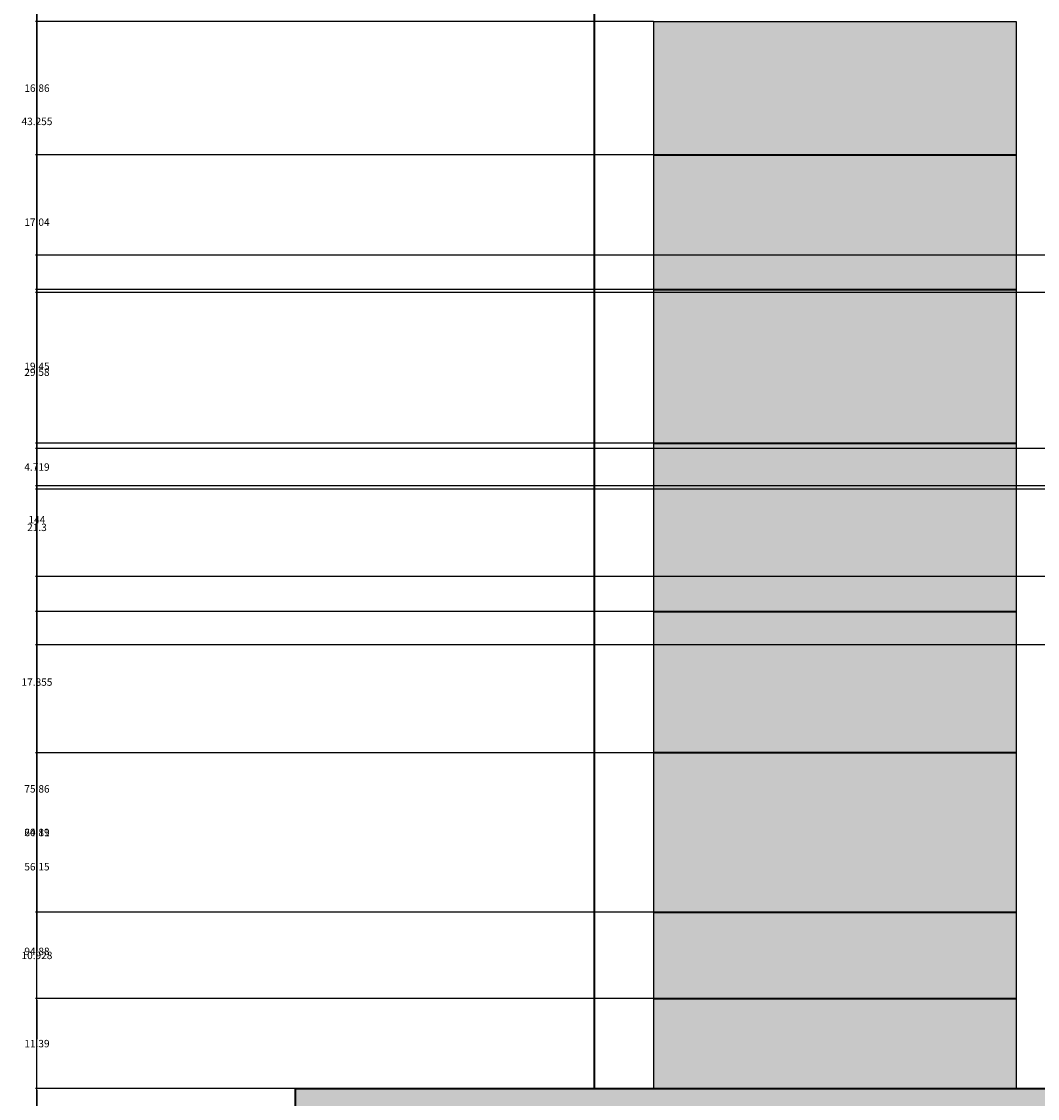
# Model space of a CAD drawing. Units: inches. Extents: x -5 to 714, y 84 to 644.
# Tile 2 of 20: x -5 to 124, y 200 to 336. Entities that reach past the tile are written whole.
import ezdxf

# ---------------------------------------------------------------- set-up
doc = ezdxf.new("R2010")
doc.units = ezdxf.units.IN
doc.header["$MEASUREMENT"] = 0
for name, color, linetype, lineweight in [('A-ANNO-DIMS', 2, 'Continuous', 18), ('A-ELEV', 7, 'Continuous', 35), ('A-ELEV-PATT', 8, 'Continuous', 13), ('A-GLAZ', 3, 'Continuous', 25)]:
    doc.layers.add(name, color=color, linetype=linetype, lineweight=lineweight)
doc.styles.get("Standard").update_dxf_attribs({"font": 'arial.ttf'})
doc.dimstyles.get("Standard").update_dxf_attribs({"dimtxt": 0.9375, "dimasz": 0.18, "dimexe": 0.18, "dimexo": 0.0625, "dimgap": 0.09, "dimtad": 0, "dimtih": 1, "dimtoh": 1, "dimdec": 4, "dimzin": 0, "dimdsep": 46, "dimlunit": 4, "dimtxsty": 'Standard', "dimcen": 0.09, "dimadec": 0, "dimazin": 0, "dimtfac": 1, "dimtdec": 4, "dimtofl": 0, "dimtmove": 0, "dimatfit": 3, "dimfxl": 1, "dimtolj": 1, "dimtzin": 0, "dimarcsym": 0})

# ---------------------------------------------------------------- blocks, each defined once
blk = doc.blocks.new('*D2')
at = {"layer": 'A-ANNO-DIMS', "color": 0, "lineweight": -2, "transparency": 16777216}
for p, q in [((67.93, 610.73), (-2.74, 610.73)), ((-2.56, 610.55), (-2.56, 364.53)), ((-2.56, 117.37), (-2.56, 363.39)), ((30.08, 117.19), (-2.74, 117.19))]:
    blk.add_line(p, q, dxfattribs=at)
at = {"layer": 'A-ANNO-DIMS', "color": 0, "transparency": 16777216}
for points in [[(-2.59, 610.55), (-2.53, 610.55), (-2.56, 610.73)], [(-2.59, 117.37), (-2.53, 117.37), (-2.56, 117.19)]]:
    blk.add_solid(points, dxfattribs=at)
at = {"layer": 'Defpoints', "color": 0, "transparency": 16777216}
for p in [(-2.56, 610.73), (67.99, 610.73), (30.14, 117.19)]:
    blk.add_point(p, dxfattribs=at)
at = {"layer": 'A-ANNO-DIMS', "color": 0, "transparency": 16777216, "insert": (-2.56, 363.96), "char_height": 0.938, "attachment_point": 5}
blk.add_mtext('\\A1;493.5', dxfattribs=at)
blk = doc.blocks.new('*D4')
at = {"layer": 'A-ANNO-DIMS', "color": 0, "lineweight": -2, "transparency": 16777216}
for p, q in [((30.08, 201.19), (-2.74, 201.19)), ((-2.56, 201.01), (-2.56, 171.76)), ((-2.56, 141.37), (-2.56, 170.62)), ((30.08, 141.19), (-2.74, 141.19))]:
    blk.add_line(p, q, dxfattribs=at)
at = {"layer": 'A-ANNO-DIMS', "color": 0, "transparency": 16777216}
for points in [[(-2.59, 201.01), (-2.53, 201.01), (-2.56, 201.19)], [(-2.59, 141.37), (-2.53, 141.37), (-2.56, 141.19)]]:
    blk.add_solid(points, dxfattribs=at)
at = {"layer": 'Defpoints', "color": 0, "transparency": 16777216}
for p in [(-2.56, 201.19), (30.14, 201.19), (30.14, 141.19)]:
    blk.add_point(p, dxfattribs=at)
at = {"layer": 'A-ANNO-DIMS', "color": 0, "transparency": 16777216, "insert": (-2.56, 171.19), "char_height": 0.938, "attachment_point": 5}
blk.add_mtext('\\A1;60', dxfattribs=at)
blk = doc.blocks.new('*D5')
at = {"layer": 'A-ANNO-DIMS', "color": 0, "lineweight": -2, "transparency": 16777216}
for p, q in [((67.93, 345.19), (-2.74, 345.19)), ((-2.56, 345.01), (-2.56, 273.75)), ((-2.56, 201.37), (-2.56, 272.63)), ((67.93, 201.19), (-2.74, 201.19))]:
    blk.add_line(p, q, dxfattribs=at)
at = {"layer": 'A-ANNO-DIMS', "color": 0, "transparency": 16777216}
for points in [[(-2.59, 345.01), (-2.53, 345.01), (-2.56, 345.19)], [(-2.59, 201.37), (-2.53, 201.37), (-2.56, 201.19)]]:
    blk.add_solid(points, dxfattribs=at)
at = {"layer": 'Defpoints', "color": 0, "transparency": 16777216}
for p in [(-2.56, 345.19), (67.99, 345.19), (67.99, 201.19)]:
    blk.add_point(p, dxfattribs=at)
at = {"layer": 'A-ANNO-DIMS', "color": 0, "transparency": 16777216, "insert": (-2.56, 273.19), "char_height": 0.938, "attachment_point": 5}
blk.add_mtext('\\A1;144', dxfattribs=at)
blk = doc.blocks.new('*D38')
at = {"layer": 'A-ANNO-DIMS', "color": 0, "lineweight": -2, "transparency": 16777216}
for p, q in [((75.44, 212.58), (-2.74, 212.58)), ((-2.56, 212.4), (-2.56, 207.46)), ((-2.56, 201.37), (-2.56, 206.32)), ((75.44, 201.19), (-2.74, 201.19))]:
    blk.add_line(p, q, dxfattribs=at)
at = {"layer": 'A-ANNO-DIMS', "color": 0, "transparency": 16777216}
for points in [[(-2.59, 212.4), (-2.53, 212.4), (-2.56, 212.58)], [(-2.59, 201.37), (-2.53, 201.37), (-2.56, 201.19)]]:
    blk.add_solid(points, dxfattribs=at)
at = {"layer": 'Defpoints', "color": 0, "transparency": 16777216}
for p in [(-2.56, 212.58), (75.5, 212.58), (75.5, 201.19)]:
    blk.add_point(p, dxfattribs=at)
at = {"layer": 'A-ANNO-DIMS', "color": 0, "transparency": 16777216, "insert": (-2.56, 206.89), "char_height": 0.938, "attachment_point": 5}
blk.add_mtext('\\A1;11.39', dxfattribs=at)
blk = doc.blocks.new('*D39')
at = {"layer": 'A-ANNO-DIMS', "color": 0, "lineweight": -2, "transparency": 16777216}
for p, q in [((75.44, 223.51), (-2.74, 223.51)), ((-2.56, 223.33), (-2.56, 218.62)), ((-2.56, 212.76), (-2.56, 217.48)), ((75.44, 212.58), (-2.74, 212.58))]:
    blk.add_line(p, q, dxfattribs=at)
at = {"layer": 'A-ANNO-DIMS', "color": 0, "transparency": 16777216}
for points in [[(-2.59, 223.33), (-2.53, 223.33), (-2.56, 223.51)], [(-2.59, 212.76), (-2.53, 212.76), (-2.56, 212.58)]]:
    blk.add_solid(points, dxfattribs=at)
at = {"layer": 'Defpoints', "color": 0, "transparency": 16777216}
for p in [(-2.56, 223.51), (75.5, 223.51), (75.5, 212.58)]:
    blk.add_point(p, dxfattribs=at)
at = {"layer": 'A-ANNO-DIMS', "color": 0, "transparency": 16777216, "insert": (-2.56, 218.05), "char_height": 0.938, "attachment_point": 5}
blk.add_mtext('\\A1;10.928', dxfattribs=at)
blk = doc.blocks.new('*D40')
at = {"layer": 'A-ANNO-DIMS', "color": 0, "lineweight": -2, "transparency": 16777216}
for p, q in [((75.44, 243.7), (-2.74, 243.7)), ((-2.56, 243.52), (-2.56, 234.17)), ((-2.56, 223.69), (-2.56, 233.04)), ((75.44, 223.51), (-2.74, 223.51))]:
    blk.add_line(p, q, dxfattribs=at)
at = {"layer": 'A-ANNO-DIMS', "color": 0, "transparency": 16777216}
for points in [[(-2.59, 243.52), (-2.53, 243.52), (-2.56, 243.7)], [(-2.59, 223.69), (-2.53, 223.69), (-2.56, 223.51)]]:
    blk.add_solid(points, dxfattribs=at)
at = {"layer": 'Defpoints', "color": 0, "transparency": 16777216}
for p in [(-2.56, 243.7), (75.5, 243.7), (75.5, 223.51)]:
    blk.add_point(p, dxfattribs=at)
at = {"layer": 'A-ANNO-DIMS', "color": 0, "transparency": 16777216, "insert": (-2.56, 233.61), "char_height": 0.938, "attachment_point": 5}
blk.add_mtext('\\A1;20.19', dxfattribs=at)
blk = doc.blocks.new('*D41')
at = {"layer": 'A-ANNO-DIMS', "color": 0, "lineweight": -2, "transparency": 16777216}
for p, q in [((75.44, 261.56), (-2.74, 261.56)), ((-2.56, 261.38), (-2.56, 253.2)), ((-2.56, 243.88), (-2.56, 252.06)), ((75.44, 243.7), (-2.74, 243.7))]:
    blk.add_line(p, q, dxfattribs=at)
at = {"layer": 'A-ANNO-DIMS', "color": 0, "transparency": 16777216}
for points in [[(-2.59, 261.38), (-2.53, 261.38), (-2.56, 261.56)], [(-2.59, 243.88), (-2.53, 243.88), (-2.56, 243.7)]]:
    blk.add_solid(points, dxfattribs=at)
at = {"layer": 'Defpoints', "color": 0, "transparency": 16777216}
for p in [(-2.56, 261.56), (75.5, 261.56), (75.5, 243.7)]:
    blk.add_point(p, dxfattribs=at)
at = {"layer": 'A-ANNO-DIMS', "color": 0, "transparency": 16777216, "insert": (-2.56, 252.63), "char_height": 0.938, "attachment_point": 5}
blk.add_mtext('\\A1;17.855', dxfattribs=at)
blk = doc.blocks.new('*D42')
at = {"layer": 'A-ANNO-DIMS', "color": 0, "lineweight": -2, "transparency": 16777216}
for p, q in [((75.44, 282.86), (-2.74, 282.86)), ((-2.56, 282.68), (-2.56, 272.77)), ((-2.56, 261.74), (-2.56, 271.64)), ((75.44, 261.56), (-2.74, 261.56))]:
    blk.add_line(p, q, dxfattribs=at)
at = {"layer": 'A-ANNO-DIMS', "color": 0, "transparency": 16777216}
for points in [[(-2.59, 282.68), (-2.53, 282.68), (-2.56, 282.86)], [(-2.59, 261.74), (-2.53, 261.74), (-2.56, 261.56)]]:
    blk.add_solid(points, dxfattribs=at)
at = {"layer": 'Defpoints', "color": 0, "transparency": 16777216}
for p in [(-2.56, 282.86), (75.5, 282.86), (75.5, 261.56)]:
    blk.add_point(p, dxfattribs=at)
at = {"layer": 'A-ANNO-DIMS', "color": 0, "transparency": 16777216, "insert": (-2.56, 272.21), "char_height": 0.938, "attachment_point": 5}
blk.add_mtext('\\A1;21.3', dxfattribs=at)
blk = doc.blocks.new('*D43')
at = {"layer": 'A-ANNO-DIMS', "color": 0, "lineweight": -2, "transparency": 16777216}
for p, q in [((75.44, 302.3), (-2.74, 302.3)), ((-2.56, 302.12), (-2.56, 293.15)), ((-2.56, 283.04), (-2.56, 292.01)), ((75.44, 282.86), (-2.74, 282.86))]:
    blk.add_line(p, q, dxfattribs=at)
at = {"layer": 'A-ANNO-DIMS', "color": 0, "transparency": 16777216}
for points in [[(-2.59, 302.12), (-2.53, 302.12), (-2.56, 302.3)], [(-2.59, 283.04), (-2.53, 283.04), (-2.56, 282.86)]]:
    blk.add_solid(points, dxfattribs=at)
at = {"layer": 'Defpoints', "color": 0, "transparency": 16777216}
for p in [(-2.56, 302.3), (75.5, 302.3), (75.5, 282.86)]:
    blk.add_point(p, dxfattribs=at)
at = {"layer": 'A-ANNO-DIMS', "color": 0, "transparency": 16777216, "insert": (-2.56, 292.58), "char_height": 0.938, "attachment_point": 5}
blk.add_mtext('\\A1;19.45', dxfattribs=at)
blk = doc.blocks.new('*D44')
at = {"layer": 'A-ANNO-DIMS', "color": 0, "lineweight": -2, "transparency": 16777216}
for p, q in [((75.44, 319.34), (-2.74, 319.34)), ((-2.56, 319.16), (-2.56, 311.39)), ((-2.56, 302.48), (-2.56, 310.26)), ((75.44, 302.3), (-2.74, 302.3))]:
    blk.add_line(p, q, dxfattribs=at)
at = {"layer": 'A-ANNO-DIMS', "color": 0, "transparency": 16777216}
for points in [[(-2.59, 319.16), (-2.53, 319.16), (-2.56, 319.34)], [(-2.59, 302.48), (-2.53, 302.48), (-2.56, 302.3)]]:
    blk.add_solid(points, dxfattribs=at)
at = {"layer": 'Defpoints', "color": 0, "transparency": 16777216}
for p in [(-2.56, 319.34), (75.5, 319.34), (75.5, 302.3)]:
    blk.add_point(p, dxfattribs=at)
at = {"layer": 'A-ANNO-DIMS', "color": 0, "transparency": 16777216, "insert": (-2.56, 310.82), "char_height": 0.938, "attachment_point": 5}
blk.add_mtext('\\A1;17.04', dxfattribs=at)
blk = doc.blocks.new('*D45')
at = {"layer": 'A-ANNO-DIMS', "color": 0, "lineweight": -2, "transparency": 16777216}
for p, q in [((75.44, 336.21), (-2.74, 336.21)), ((-2.56, 336.03), (-2.56, 328.34)), ((-2.56, 319.52), (-2.56, 327.21)), ((75.44, 319.34), (-2.74, 319.34))]:
    blk.add_line(p, q, dxfattribs=at)
at = {"layer": 'A-ANNO-DIMS', "color": 0, "transparency": 16777216}
for points in [[(-2.59, 336.03), (-2.53, 336.03), (-2.56, 336.21)], [(-2.59, 319.52), (-2.53, 319.52), (-2.56, 319.34)]]:
    blk.add_solid(points, dxfattribs=at)
at = {"layer": 'Defpoints', "color": 0, "transparency": 16777216}
for p in [(-2.56, 336.21), (75.5, 336.21), (75.5, 319.34)]:
    blk.add_point(p, dxfattribs=at)
at = {"layer": 'A-ANNO-DIMS', "color": 0, "transparency": 16777216, "insert": (-2.56, 327.78), "char_height": 0.938, "attachment_point": 5}
blk.add_mtext('\\A1;16.86', dxfattribs=at)
blk = doc.blocks.new('*D50')
at = {"layer": 'A-ANNO-DIMS', "color": 0, "lineweight": -2, "transparency": 16777216}
for p, q in [((200.67, 345.19), (-2.74, 345.19)), ((-2.56, 345.01), (-2.56, 324.13)), ((-2.56, 302.12), (-2.56, 323)), ((200.67, 301.94), (-2.74, 301.94))]:
    blk.add_line(p, q, dxfattribs=at)
at = {"layer": 'A-ANNO-DIMS', "color": 0, "transparency": 16777216}
for points in [[(-2.59, 345.01), (-2.53, 345.01), (-2.56, 345.19)], [(-2.59, 302.12), (-2.53, 302.12), (-2.56, 301.94)]]:
    blk.add_solid(points, dxfattribs=at)
at = {"layer": 'Defpoints', "color": 0, "transparency": 16777216}
for p in [(-2.56, 345.19), (200.74, 345.19), (200.74, 301.94)]:
    blk.add_point(p, dxfattribs=at)
at = {"layer": 'A-ANNO-DIMS', "color": 0, "transparency": 16777216, "insert": (-2.56, 323.57), "char_height": 0.938, "attachment_point": 5}
blk.add_mtext('\\A1;43.255', dxfattribs=at)
blk = doc.blocks.new('*D56')
at = {"layer": 'A-ANNO-DIMS', "color": 0, "lineweight": -2, "transparency": 16777216}
for p, q in [((578.03, 277.05), (-2.74, 277.05)), ((-2.56, 276.87), (-2.56, 239.69)), ((-2.56, 201.37), (-2.56, 238.55)), ((578.03, 201.19), (-2.74, 201.19))]:
    blk.add_line(p, q, dxfattribs=at)
at = {"layer": 'A-ANNO-DIMS', "color": 0, "transparency": 16777216}
for points in [[(-2.59, 276.87), (-2.53, 276.87), (-2.56, 277.05)], [(-2.59, 201.37), (-2.53, 201.37), (-2.56, 201.19)]]:
    blk.add_solid(points, dxfattribs=at)
at = {"layer": 'Defpoints', "color": 0, "transparency": 16777216}
for p in [(-2.56, 277.05), (578.09, 277.05), (578.09, 201.19)]:
    blk.add_point(p, dxfattribs=at)
at = {"layer": 'A-ANNO-DIMS', "color": 0, "transparency": 16777216, "insert": (-2.56, 239.12), "char_height": 0.938, "attachment_point": 5}
blk.add_mtext('\\A1;75.86', dxfattribs=at)
blk = doc.blocks.new('*D57')
at = {"layer": 'A-ANNO-DIMS', "color": 0, "lineweight": -2, "transparency": 16777216}
for p, q in [((578.03, 306.63), (-2.74, 306.63)), ((-2.56, 306.45), (-2.56, 292.41)), ((-2.56, 277.23), (-2.56, 291.27)), ((578.03, 277.05), (-2.74, 277.05))]:
    blk.add_line(p, q, dxfattribs=at)
at = {"layer": 'A-ANNO-DIMS', "color": 0, "transparency": 16777216}
for points in [[(-2.59, 306.45), (-2.53, 306.45), (-2.56, 306.63)], [(-2.59, 277.23), (-2.53, 277.23), (-2.56, 277.05)]]:
    blk.add_solid(points, dxfattribs=at)
at = {"layer": 'Defpoints', "color": 0, "transparency": 16777216}
for p in [(578.09, 306.63), (-2.56, 277.05), (578.09, 277.05)]:
    blk.add_point(p, dxfattribs=at)
at = {"layer": 'A-ANNO-DIMS', "color": 0, "transparency": 16777216, "insert": (-2.56, 291.84), "char_height": 0.938, "attachment_point": 5}
blk.add_mtext('\\A1;29.58', dxfattribs=at)
blk = doc.blocks.new('*D59')
at = {"layer": 'A-ANNO-DIMS', "color": 0, "lineweight": -2, "transparency": 16777216}
for p, q in [((593.37, 282.2), (-2.74, 282.2)), ((-2.56, 282.02), (-2.56, 280.41)), ((-2.56, 277.66), (-2.56, 279.27)), ((593.37, 277.48), (-2.74, 277.48))]:
    blk.add_line(p, q, dxfattribs=at)
at = {"layer": 'A-ANNO-DIMS', "color": 0, "transparency": 16777216}
for points in [[(-2.59, 282.02), (-2.53, 282.02), (-2.56, 282.2)], [(-2.59, 277.66), (-2.53, 277.66), (-2.56, 277.48)]]:
    blk.add_solid(points, dxfattribs=at)
at = {"layer": 'Defpoints', "color": 0, "transparency": 16777216}
for p in [(-2.56, 282.2), (593.43, 282.2), (593.43, 277.48)]:
    blk.add_point(p, dxfattribs=at)
at = {"layer": 'A-ANNO-DIMS', "color": 0, "transparency": 16777216, "insert": (-2.56, 279.84), "char_height": 0.938, "attachment_point": 5}
blk.add_mtext('\\A1;4.719', dxfattribs=at)
blk = doc.blocks.new('*D65')
at = {"layer": 'A-ANNO-DIMS', "color": 0, "lineweight": -2, "transparency": 16777216}
for p, q in [((325.77, 266), (-2.74, 266)), ((-2.56, 265.82), (-2.56, 219.13)), ((-2.56, 171.3), (-2.56, 217.99)), ((325.77, 171.12), (-2.74, 171.12))]:
    blk.add_line(p, q, dxfattribs=at)
at = {"layer": 'A-ANNO-DIMS', "color": 0, "transparency": 16777216}
for points in [[(-2.59, 265.82), (-2.53, 265.82), (-2.56, 266)], [(-2.59, 171.3), (-2.53, 171.3), (-2.56, 171.12)]]:
    blk.add_solid(points, dxfattribs=at)
at = {"layer": 'Defpoints', "color": 0, "transparency": 16777216}
for p in [(-2.56, 266), (325.83, 266), (325.83, 171.12)]:
    blk.add_point(p, dxfattribs=at)
at = {"layer": 'A-ANNO-DIMS', "color": 0, "transparency": 16777216, "insert": (-2.56, 218.56), "char_height": 0.938, "attachment_point": 5}
blk.add_mtext('\\A1;94.88', dxfattribs=at)
blk = doc.blocks.new('*D71')
at = {"layer": 'A-ANNO-DIMS', "color": 0, "lineweight": -2, "transparency": 16777216}
for p, q in [((537.12, 257.34), (-2.74, 257.34)), ((-2.56, 257.16), (-2.56, 229.83)), ((-2.56, 201.37), (-2.56, 228.7)), ((537.12, 201.19), (-2.74, 201.19))]:
    blk.add_line(p, q, dxfattribs=at)
at = {"layer": 'A-ANNO-DIMS', "color": 0, "transparency": 16777216}
for points in [[(-2.59, 257.16), (-2.53, 257.16), (-2.56, 257.34)], [(-2.59, 201.37), (-2.53, 201.37), (-2.56, 201.19)]]:
    blk.add_solid(points, dxfattribs=at)
at = {"layer": 'Defpoints', "color": 0, "transparency": 16777216}
for p in [(-2.56, 257.34), (537.18, 257.34), (537.18, 201.19)]:
    blk.add_point(p, dxfattribs=at)
at = {"layer": 'A-ANNO-DIMS', "color": 0, "transparency": 16777216, "insert": (-2.56, 229.27), "char_height": 0.938, "attachment_point": 5}
blk.add_mtext('\\A1;56.15', dxfattribs=at)
blk = doc.blocks.new('*D72')
at = {"layer": 'A-ANNO-DIMS', "color": 0, "lineweight": -2, "transparency": 16777216}
for p, q in [((493.71, 266), (-2.74, 266)), ((-2.56, 265.82), (-2.56, 234.17)), ((-2.56, 201.37), (-2.56, 233.03)), ((493.71, 201.19), (-2.74, 201.19))]:
    blk.add_line(p, q, dxfattribs=at)
at = {"layer": 'A-ANNO-DIMS', "color": 0, "transparency": 16777216}
for points in [[(-2.59, 265.82), (-2.53, 265.82), (-2.56, 266)], [(-2.59, 201.37), (-2.53, 201.37), (-2.56, 201.19)]]:
    blk.add_solid(points, dxfattribs=at)
at = {"layer": 'Defpoints', "color": 0, "transparency": 16777216}
for p in [(-2.56, 266), (493.78, 266), (493.78, 201.19)]:
    blk.add_point(p, dxfattribs=at)
at = {"layer": 'A-ANNO-DIMS', "color": 0, "transparency": 16777216, "insert": (-2.56, 233.6), "char_height": 0.938, "attachment_point": 5}
blk.add_mtext('\\A1;64.81', dxfattribs=at)
blk = doc.blocks.new('*D82')
at = {"layer": 'A-ANNO-DIMS', "color": 0, "lineweight": -2, "transparency": 16777216}
for p, q in [((263.37, 201.19), (-2.74, 201.19)), ((-2.56, 201.01), (-2.56, 177.22)), ((-2.56, 152.3), (-2.56, 176.09)), ((263.37, 152.12), (-2.74, 152.12))]:
    blk.add_line(p, q, dxfattribs=at)
at = {"layer": 'A-ANNO-DIMS', "color": 0, "transparency": 16777216}
for points in [[(-2.59, 201.01), (-2.53, 201.01), (-2.56, 201.19)], [(-2.59, 152.3), (-2.53, 152.3), (-2.56, 152.12)]]:
    blk.add_solid(points, dxfattribs=at)
at = {"layer": 'Defpoints', "color": 0, "transparency": 16777216}
for p in [(-2.56, 201.19), (263.43, 201.19), (263.43, 152.12)]:
    blk.add_point(p, dxfattribs=at)
at = {"layer": 'A-ANNO-DIMS', "color": 0, "transparency": 16777216, "insert": (-2.56, 176.66), "char_height": 0.938, "attachment_point": 5}
blk.add_mtext('\\A1;49.08', dxfattribs=at)

msp = doc.modelspace()

# ---------------------------------------------------------------- hatches: boundary and pattern name
at = {"layer": 'A-ELEV-PATT', "transparency": 33554687}
h = msp.add_hatch(color=256, dxfattribs=at)
h.dxf.hatch_style = 1
h.paths.add_polyline_path([(188.3677, 525.1928), (67.9893, 525.1928), (67.9893, 489.1928), (67.9893, 345.1928), (126.7303, 345.1928), (126.7303, 480.1709), (229.3575, 480.1709), (229.3575, 525.1928), (212.6043, 525.1928), (212.6043, 482.7164), (211.0019, 482.7164), (211.0019, 525.1928), (207.6919, 525.1928), (199.9852, 525.1928), (199.9852, 482.7164), (198.3828, 482.7164), (198.3828, 525.1928), (189.9701, 525.1928), (189.9701, 482.7164), (188.3677, 482.7164)])
h.paths.add_polyline_path([(121.3589, 336.2066), (75.5048, 336.2066), (75.5048, 319.345), (121.3589, 319.345)])
h.paths.add_polyline_path([(121.3589, 319.345), (75.5048, 319.345), (75.5048, 302.3045), (121.3589, 302.3045)])
h.paths.add_polyline_path([(121.3589, 302.3045), (75.5048, 302.3045), (75.5048, 282.8561), (121.3589, 282.8561)])
h.paths.add_polyline_path([(121.3589, 282.8561), (75.5048, 282.8561), (75.5048, 261.5556), (121.3589, 261.5556)])
h.paths.add_polyline_path([(121.3589, 261.5556), (75.5048, 261.5556), (75.5048, 243.7009), (121.3589, 243.7009)])
h.paths.add_polyline_path([(121.3589, 243.7009), (75.5048, 243.7009), (75.5048, 223.5117), (121.3589, 223.5117)])
h.paths.add_polyline_path([(121.3589, 223.5117), (75.5048, 223.5117), (75.5048, 212.5836), (121.3589, 212.5836)])
h.paths.add_polyline_path([(121.3589, 212.5836), (75.5048, 212.5836), (75.5048, 201.1928), (121.3589, 201.1928)])
h.paths.add_polyline_path([(179.9335, 201.1928), (30.1395, 201.1928), (30.1395, 198.7054), (179.9335, 198.7054)])
h.paths.add_polyline_path([(187.6349, 201.1928), (179.9335, 201.1928), (179.9335, 198.7054), (179.9335, 141.1928), (269.2446, 141.1928), (269.2446, 201.1928), (263.4349, 201.1928), (263.4349, 152.1176), (187.6349, 152.1176)])
h.paths.add_polyline_path([(269.2446, 277.0513), (269.2446, 287.501), (269.2446, 306.6286), (578.0915, 306.6286), (578.0915, 201.1928), (593.428, 201.1928), (593.428, 315.0968), (584.4202, 315.0968), (259.0665, 315.0968), (259.0665, 201.1928), (263.4349, 201.1928), (269.2446, 201.1928)])

# ---------------------------------------------------------------- linework, layer by layer
at = {"layer": 'A-ELEV'}
for p, q in [((67.9893, 201.1928), (67.9893, 345.1928)), ((75.5048, 319.345), (121.3589, 319.345)), ((75.5048, 302.3045), (121.3589, 302.3045)), ((75.5048, 282.8561), (121.3589, 282.8561)), ((75.5048, 261.5556), (121.3589, 261.5556)), ((75.5048, 243.7009), (121.3589, 243.7009)), ((75.5048, 223.5117), (121.3589, 223.5117)), ((75.5048, 212.5836), (121.3589, 212.5836)), ((30.1395, 141.1928), (30.1395, 201.1928)), ((30.1395, 201.1928), (545.1065, 201.1928))]:
    msp.add_line(p, q, dxfattribs=at)
at = {"layer": 'A-GLAZ'}
msp.add_lwpolyline([(75.5048, 336.2066), (121.3589, 336.2066), (121.3589, 201.1928), (75.5048, 201.1928)], close=True, dxfattribs=at)

# ---------------------------------------------------------------- dimensions: what is measured, and where the dimension line sits
at = {"layer": 'A-ANNO-DIMS'}
for base, p1, p2, override, picture, middle in [((-2.5605, 610.7276), (30.1395, 117.1928), (67.9893, 610.7276), {"dimdec": 1, "dimlfac": 1, "dimrnd": 0, "dimzin": 0, "dimdsep": 46, "dimlunit": 2}, '*D2', (-2.5605, 363.9602)), ((-2.5605, 345.1928), (200.7361, 301.9374), (200.7361, 345.1928), {"dimdec": 3, "dimlfac": 1, "dimrnd": 0, "dimzin": 0, "dimdsep": 46, "dimlunit": 2}, '*D50', (-2.5605, 323.5651)), ((-2.5605, 345.1928), (67.9893, 201.1928), (67.9893, 345.1928), {"dimdec": 0, "dimlfac": 1, "dimrnd": 0, "dimzin": 0, "dimdsep": 46, "dimlunit": 2}, '*D5', (-2.5605, 273.1928)), ((-2.5605, 336.2066), (75.5048, 319.345), (75.5048, 336.2066), {"dimdec": 2, "dimlfac": 1, "dimrnd": 0, "dimzin": 0, "dimdsep": 46, "dimlunit": 2}, '*D45', (-2.5605, 327.7758)), ((-2.5605, 319.345), (75.5048, 302.3045), (75.5048, 319.345), {"dimdec": 2, "dimlfac": 1, "dimrnd": 0, "dimzin": 0, "dimdsep": 46, "dimlunit": 2}, '*D44', (-2.5605, 310.8247)), ((-2.5605, 277.0513), (578.0915, 306.6286), (578.0915, 277.0513), {"dimdec": 2, "dimlfac": 1, "dimrnd": 0, "dimzin": 0, "dimdsep": 46, "dimlunit": 2}, '*D57', (-2.5605, 291.84)), ((-2.5605, 302.3045), (75.5048, 282.8561), (75.5048, 302.3045), {"dimdec": 2, "dimlfac": 1, "dimrnd": 0, "dimzin": 0, "dimdsep": 46, "dimlunit": 2}, '*D43', (-2.5605, 292.5803)), ((-2.5605, 282.1969), (593.428, 277.4776), (593.428, 282.1969), {"dimdec": 3, "dimlfac": 1, "dimrnd": 0, "dimzin": 0, "dimdsep": 46, "dimlunit": 2}, '*D59', (-2.5605, 279.8372)), ((-2.5605, 282.8561), (75.5048, 261.5556), (75.5048, 282.8561), {"dimdec": 1, "dimlfac": 1, "dimrnd": 0, "dimzin": 0, "dimdsep": 46, "dimlunit": 2}, '*D42', (-2.5605, 272.2058)), ((-2.5605, 277.0513), (578.0915, 201.1928), (578.0915, 277.0513), {"dimdec": 2, "dimlfac": 1, "dimrnd": 0, "dimzin": 0, "dimdsep": 46, "dimlunit": 2}, '*D56', (-2.5605, 239.1221)), ((-2.5605, 266.0021), (325.8305, 171.1197), (325.8305, 266.0021), {"dimdec": 2, "dimlfac": 1, "dimrnd": 0, "dimzin": 0, "dimdsep": 46, "dimlunit": 2}, '*D65', (-2.5605, 218.5609)), ((-2.5605, 266.0021), (493.7771, 201.1928), (493.7771, 266.0021), {"dimdec": 2, "dimlfac": 1, "dimrnd": 0, "dimzin": 0, "dimdsep": 46, "dimlunit": 2}, '*D72', (-2.5605, 233.5974)), ((-2.5605, 261.5556), (75.5048, 243.7009), (75.5048, 261.5556), {"dimdec": 3, "dimlfac": 1, "dimrnd": 0, "dimzin": 0, "dimdsep": 46, "dimlunit": 2}, '*D41', (-2.5605, 252.6282)), ((-2.5605, 257.3379), (537.1779, 201.1928), (537.1779, 257.3379), {"dimdec": 2, "dimlfac": 1, "dimrnd": 0, "dimzin": 0, "dimdsep": 46, "dimlunit": 2}, '*D71', (-2.5605, 229.2653)), ((-2.5605, 243.7009), (75.5048, 223.5117), (75.5048, 243.7009), {"dimdec": 2, "dimlfac": 1, "dimrnd": 0, "dimzin": 0, "dimdsep": 46, "dimlunit": 2}, '*D40', (-2.5605, 233.6063)), ((-2.5605, 223.5117), (75.5048, 212.5836), (75.5048, 223.5117), {"dimdec": 3, "dimlfac": 1, "dimrnd": 0, "dimzin": 0, "dimdsep": 46, "dimlunit": 2}, '*D39', (-2.5605, 218.0476)), ((-2.5605, 212.5836), (75.5048, 201.1928), (75.5048, 212.5836), {"dimdec": 2, "dimlfac": 1, "dimrnd": 0, "dimzin": 0, "dimdsep": 46, "dimlunit": 2}, '*D38', (-2.5605, 206.8882)), ((-2.5605, 201.1928), (263.4349, 152.1176), (263.4349, 201.1928), {"dimdec": 2, "dimlfac": 1, "dimrnd": 0, "dimzin": 0, "dimdsep": 46, "dimlunit": 2}, '*D82', (-2.5605, 176.6552)), ((-2.5605, 201.1928), (30.1395, 141.1928), (30.1395, 201.1928), {"dimdec": 0, "dimlfac": 1, "dimrnd": 0, "dimzin": 0, "dimdsep": 46, "dimlunit": 2}, '*D4', (-2.5605, 171.1928))]:
    dim = msp.add_linear_dim(base=base, p1=p1, p2=p2, angle=90, dimstyle='Standard', override=override, dxfattribs=at)
    dim.commit()
    dim.dimension.update_dxf_attribs({"geometry": picture, "text_midpoint": middle})

doc.saveas('drawing.dxf')
